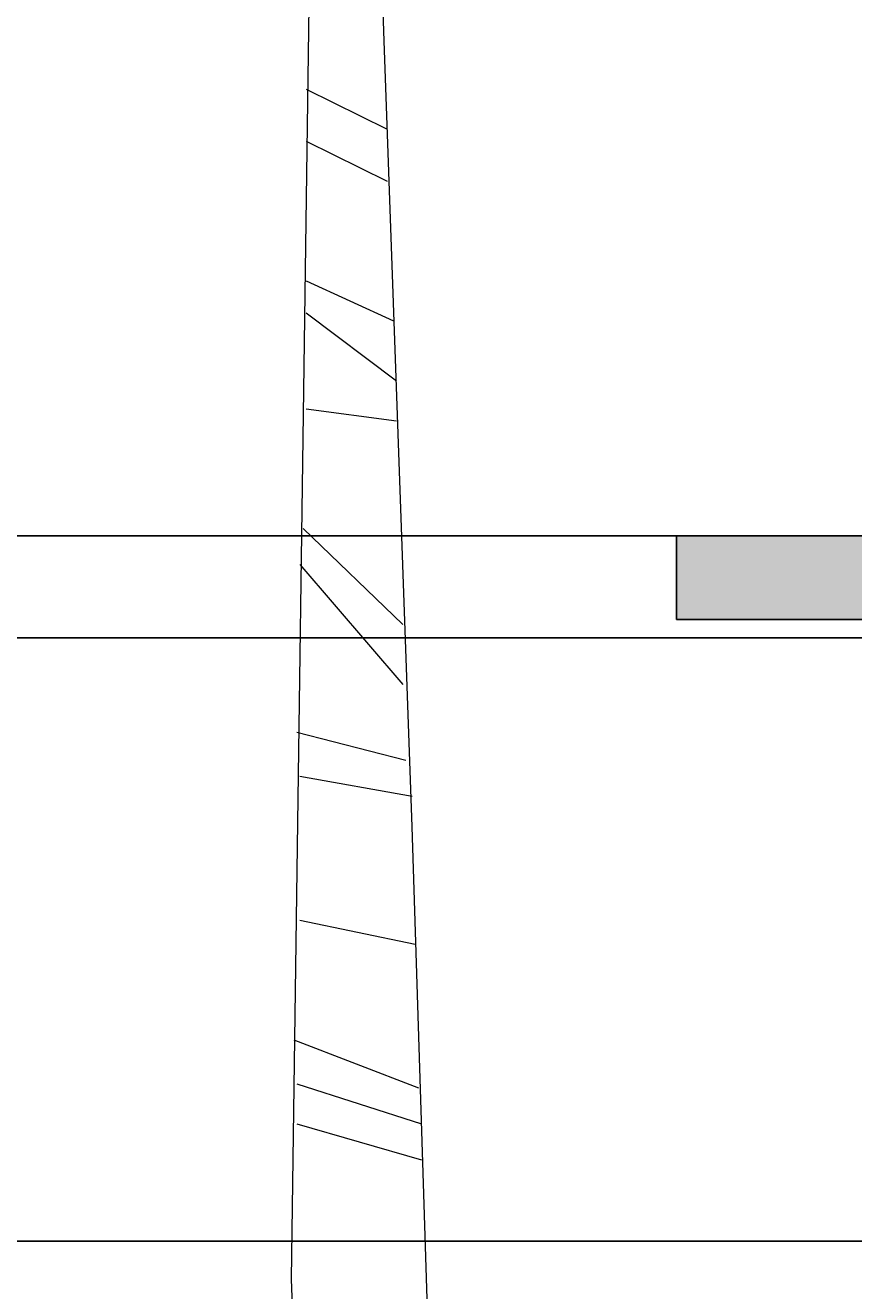
# Model space of a CAD drawing. Units: inches. Extents: x 37 to 824, y -700 to 234.
# Tile 3 of 77: x 110 to 160, y -535 to -459. Entities that reach past the tile are written whole.
import ezdxf

# ---------------------------------------------------------------- set-up
doc = ezdxf.new("R2010")
doc.units = ezdxf.units.IN
doc.header["$MEASUREMENT"] = 0
for name, color, linetype, lineweight in [('A-ANNO-DIMS', 2, 'Continuous', 18), ('A-ELEV', 3, 'Continuous', 25), ('A-ELEV-PATT', 8, 'Continuous', 13), ('A-SITE-PLNT', 3, 'Continuous', 13)]:
    doc.layers.add(name, color=color, linetype=linetype, lineweight=lineweight)
doc.styles.get("Standard").update_dxf_attribs({"font": 'arial.ttf'})
doc.dimstyles.get("Standard").update_dxf_attribs({"dimtxt": 0.18, "dimasz": 0.18, "dimexe": 0.18, "dimexo": 0.0625, "dimgap": 0.09, "dimtad": 0, "dimtih": 1, "dimtoh": 1, "dimdec": 1, "dimzin": 0, "dimdsep": 46, "dimlunit": 4, "dimtxsty": 'Standard', "dimcen": 0.09, "dimadec": 0, "dimazin": 0, "dimtfac": 1, "dimtdec": 1, "dimtofl": 0, "dimtmove": 0, "dimatfit": 3, "dimfxl": 1, "dimtolj": 1, "dimtzin": 0, "dimarcsym": 0})

# ---------------------------------------------------------------- blocks, each defined once
blk = doc.blocks.new('*U34')
for p, q in [((-4.081, 140.645), (0.753, 138.261)), ((-4.081, 137.547), (0.753, 135.163)), ((-4.081, 129.205), (1.124, 126.821)), ((-4.081, 127.298), (1.31, 123.246)), ((-4.081, 121.578), (1.31, 120.863)), ((-4.267, 114.428), (1.682, 108.708)), ((-4.453, 112.283), (1.682, 105.133)), ((-4.639, 102.273), (1.868, 100.604)), ((-4.453, 99.651), (2.24, 98.459)), ((-4.453, 91.071), (2.426, 89.641)), ((-4.825, 83.921), (2.612, 81.061)), ((-4.639, 81.299), (2.797, 78.916)), ((-4.639, 78.916), (2.797, 76.771))]:
    blk.add_line(p, q)
for points in [[(-2.363, 170.553), (-3.88, 148.505), (-4.988, 69.634), (-3.325, 24.869), (0, 0)], [(-0.116, 162.848), (0.554, 143.532), (2.217, 96.635), (3.88, 44.054), (7.76, 12.079), (11.64, 0)]]:
    blk.add_lwpolyline(points)
blk = doc.blocks.new('*D96')
at = {"layer": 'A-ANNO-DIMS', "color": 0, "lineweight": -2, "ltscale": 0.5, "transparency": 16777216}
for p, q in [((205.015, -489.627), (36.851, -489.627)), ((37.031, -489.807), (37.031, -492.489)), ((37.031, -495.534), (37.031, -492.853)), ((211.963, -495.714), (36.851, -495.714))]:
    blk.add_line(p, q, dxfattribs=at)
at = {"layer": 'A-ANNO-DIMS', "color": 0, "ltscale": 0.5, "transparency": 16777216}
for points in [[(37.001, -489.807), (37.061, -489.807), (37.031, -489.627)], [(37.001, -495.534), (37.061, -495.534), (37.031, -495.714)]]:
    blk.add_solid(points, dxfattribs=at)
at = {"layer": 'Defpoints', "color": 0, "ltscale": 0.5, "transparency": 16777216}
for p in [(205.077, -489.627), (37.031, -495.714), (212.025, -495.714)]:
    blk.add_point(p, dxfattribs=at)
at = {"layer": 'A-ANNO-DIMS', "color": 0, "ltscale": 0.5, "transparency": 16777216, "insert": (37.031, -492.671), "char_height": 0.18, "attachment_point": 5}
blk.add_mtext('\\A1;0\'-6"', dxfattribs=at)
blk = doc.blocks.new('*D97')
at = {"layer": 'A-ANNO-DIMS', "color": 0, "lineweight": -2, "ltscale": 0.5, "transparency": 16777216}
for p, q in [((211.963, -495.714), (36.851, -495.714)), ((37.031, -495.894), (37.031, -513.532)), ((37.031, -531.534), (37.031, -513.896)), ((211.963, -531.714), (36.851, -531.714))]:
    blk.add_line(p, q, dxfattribs=at)
at = {"layer": 'A-ANNO-DIMS', "color": 0, "ltscale": 0.5, "transparency": 16777216}
for points in [[(37.001, -495.894), (37.061, -495.894), (37.031, -495.714)], [(37.001, -531.534), (37.061, -531.534), (37.031, -531.714)]]:
    blk.add_solid(points, dxfattribs=at)
at = {"layer": 'Defpoints', "color": 0, "ltscale": 0.5, "transparency": 16777216}
for p in [(212.025, -495.714), (37.031, -531.714), (212.025, -531.714)]:
    blk.add_point(p, dxfattribs=at)
at = {"layer": 'A-ANNO-DIMS', "color": 0, "ltscale": 0.5, "transparency": 16777216, "insert": (37.031, -513.714), "char_height": 0.18, "attachment_point": 5}
blk.add_mtext('\\A1;3\'-0"', dxfattribs=at)

msp = doc.modelspace()

# ---------------------------------------------------------------- hatches: boundary and pattern name
at = {"layer": 'A-ELEV-PATT', "ltscale": 0.5}
h = msp.add_hatch(color=256, dxfattribs=at)
h.dxf.hatch_style = 1
h.paths.add_polyline_path([(440.077, -489.627), (428.077, -489.627), (428.077, -494.627), (440.077, -494.627)])
h.paths.add_polyline_path([(161.077, -489.627), (149.077, -489.627), (149.077, -494.627), (161.077, -494.627)])

# ---------------------------------------------------------------- linework, layer by layer
at = {"layer": 'A-ELEV', "ltscale": 0.5}
for p, q in [((161.077, -489.627), (149.077, -489.627)), ((149.077, -489.627), (149.077, -494.627)), ((149.077, -494.627), (161.077, -494.627))]:
    msp.add_line(p, q, dxfattribs=at)

# ---------------------------------------------------------------- block references
at = {"layer": 'A-SITE-PLNT'}
msp.add_blockref('*U34', (131.077, -603.627), dxfattribs=at)

# ---------------------------------------------------------------- dimensions: what is measured, and where the dimension line sits
at = {"layer": 'A-ANNO-DIMS', "ltscale": 0.5}
for base, p1, p2, picture, middle in [((37.031, -495.714), (205.077, -489.627), (212.025, -495.714), '*D96', (37.031, -492.671)), ((37.031, -531.714), (212.025, -495.714), (212.025, -531.714), '*D97', (37.031, -513.714))]:
    dim = msp.add_linear_dim(base=base, p1=p1, p2=p2, angle=90, dimstyle='Standard', override={"dimdec": 1, "dimlfac": 1, "dimrnd": 0, "dimzin": 1, "dimdsep": 46, "dimlunit": 4, "dimfrac": 2}, dxfattribs=at)
    dim.commit()
    dim.dimension.update_dxf_attribs({"geometry": picture, "text_midpoint": middle})

doc.saveas('drawing.dxf')
